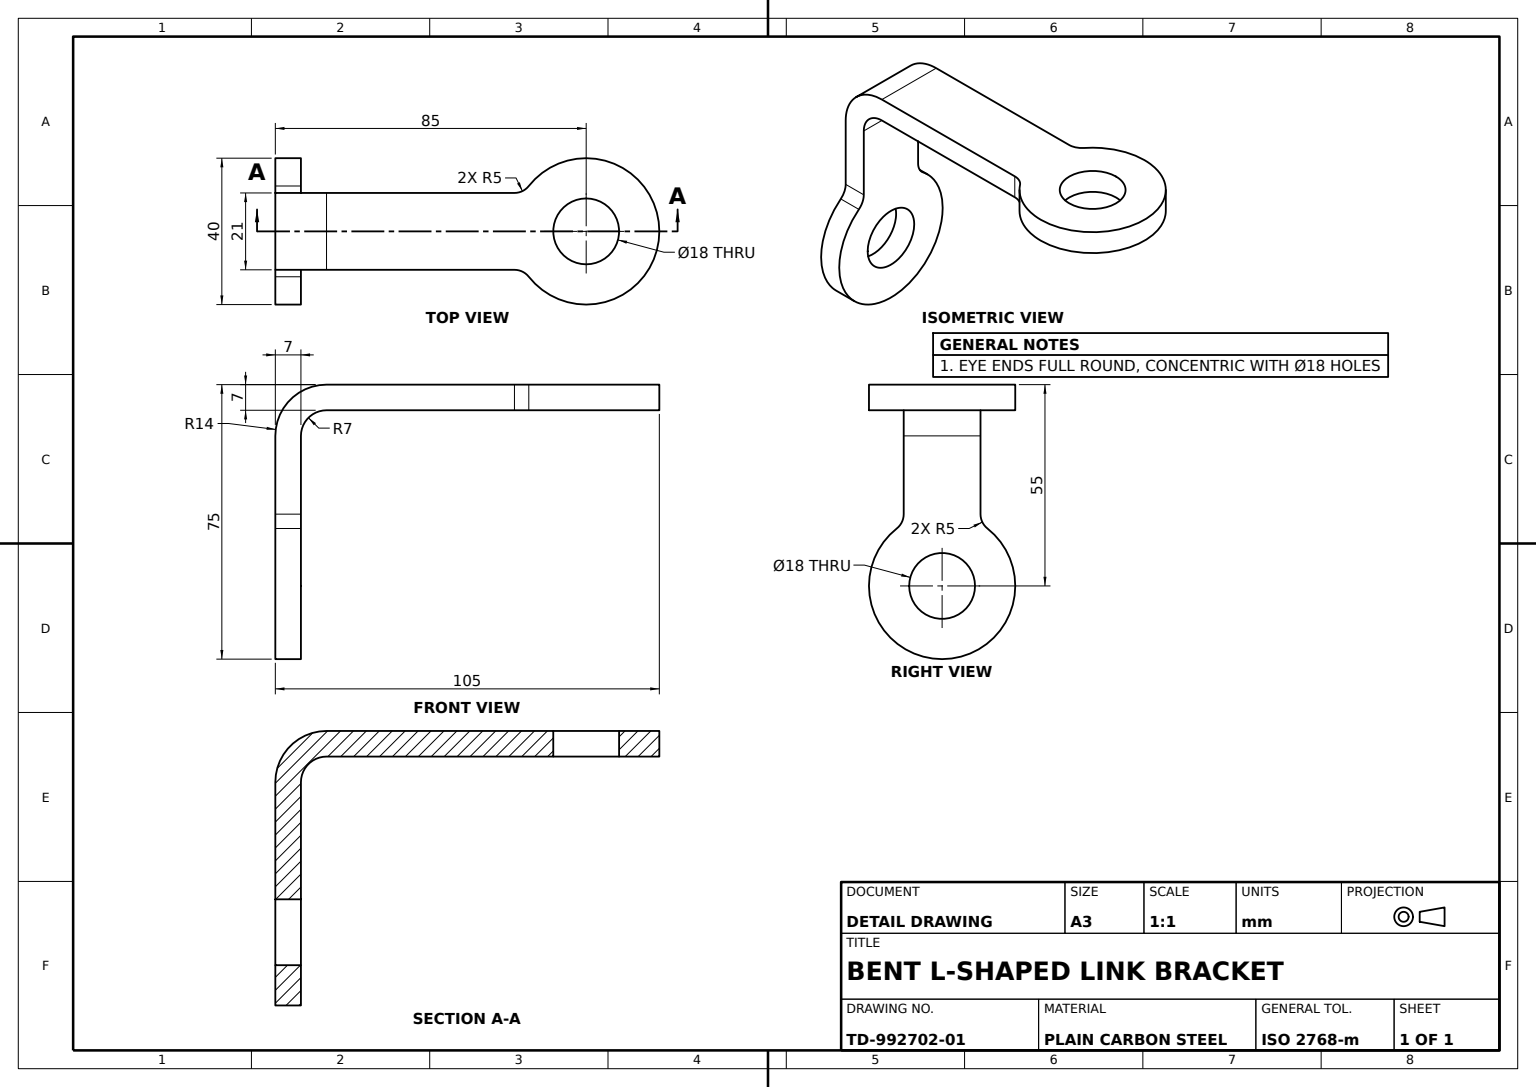
SolidWorks part; units mm, degrees
material "Plain Carbon Steel"
ref_plane "Front Plane" through (0, 0, 0) normal (0, 0, 1) x (1, 0, 0)
ref_plane "Top Plane" through (0, 0, 0) normal (0, 1, 0) x (1, 0, 0)
ref_plane "Right Plane" through (0, 0, 0) normal (1, 0, 0) x (0, 0, -1)
sketch "Horizontal Arm Profile" plane through (0, 0, 0) normal (0, 1, 0) x (1, 0, 0)
  line L0 (12.0925, 0) -> (-167.689, 0) construction
  line L1 (-17.022, 10.5) -> (-85, 10.5)
  line L2 (-17.022, -10.5) -> (-85, -10.5)
  line L3 (-85, 10.5) -> (-85, -10.5)
  circle A0 centre (0, 0) radius 9
  arc A1 (-17.022, -10.5) -> (-17.022, 10.5) centre (0, 0) ccw
  dimension "D1" = 18
  dimension "D2" = 40
  dimension "D3" = 21
  dimension "D4" = 10.5
  dimension "D5" = 85
extrude "Horizontal Arm 7mm" add sketch "Horizontal Arm Profile" against normal blind 7
ref_plane "Vertical Arm Plane" through (-85, 0, 0) normal (1, 0, 0) x (0, 0, -1)
sketch "Vertical Arm Profile" plane through (-85, 0, 0) normal (1, 0, 0) x (0, 0, -1)
  line L0 (0, 0) -> (0, -70.5902) construction
  line L1 (-10.5, 0) -> (-10.5, -37.978)
  line L2 (20, 0) -> (-20, 0) construction
  line L3 (10.5, -37.978) -> (10.5, 0)
  line L4 (-10.5, 0) -> (10.5, 0)
  circle A0 centre (0, -55) radius 9
  arc A1 (-10.5, -37.978) -> (10.5, -37.978) centre (0, -55) ccw
  dimension "D1" = 18
  dimension "D2" = 40
  dimension "D3" = 55
  dimension "D4" = 21
  dimension "D5" = 10.5
extrude "Vertical Arm 7mm" add sketch "Vertical Arm Profile" along normal blind 7
fillet "Bend Fillet R5" radius 5 4 edges at (-17.022, -3.5, -10.5) (-81.5, -37.978, -10.5) (-17.022, -3.5, 10.5) (-81.5, -37.978, 10.5)
fillet "Horizontal Arm Fillet R14" radius 14 1 edges at (-85, 0, 0)
fillet "Bend Fillet R7" radius 7 1 edges at (-78, -7, 0)
